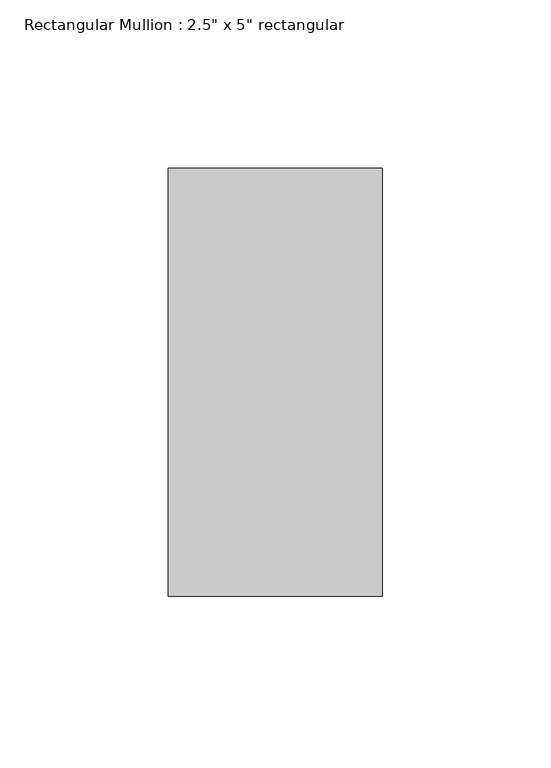
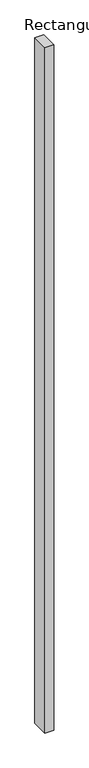
"""IFC4 building model written with IfcOpenShell, lengths in millimetres: member geometry."""

from ifc_helpers import new_model, si_unit, frame, origin, place, context, project, spatial, polyline, outline, extrude, source, transform, mapped, element, save


def member_ca95d35f(model_context):
    return source(origin(), model_context, "Body", "SweptSolid", [
        extrude(outline(polyline([(0.0, 63.5), (0.0, -63.5), (-63.5, -63.5), (-63.5, 63.5), (0.0, 63.5)])), frame((0.0, 0.0, -5295.9), z_axis=(0.0, 0.0, 1.0), x_axis=(1.0, 0.0, 0.0)), (0.0, 0.0, 1.0), 5295.9),
    ])


if __name__ == "__main__":
    model = new_model("IFC4")
    model_context = context("Model", 3, world=origin())
    ifc_project = project(units=[si_unit("LENGTHUNIT", "METRE", prefix="MILLI")], contexts=[model_context])
    site = spatial("IfcSite", under=ifc_project)
    building = spatial("IfcBuilding", under=site)
    placement = place(None, origin())
    member_shape = member_ca95d35f(model_context)
    element("IfcMember", 1, ObjectType="Rectangular Mullion : 2.5\" x 5\" rectangular", at=placement, inside=building, context=model_context, shape_type="MappedRepresentation", body=[
        mapped(member_shape, transform((0.0, 0.0, 0.0), x_axis=(1.0, 0.0, 0.0), y_axis=(0.0, 1.0, 0.0), z_axis=(0.0, 0.0, 1.0))),
    ])
    save(model, "model.ifc")

# Revit data of these elements
# Type "Rectangular Mullion : 2.5\" x 5\" rectangular"
#   built-in parameter 1007304 = 0.416667 (stored number, unit not read)
#   built-in parameter 1007301 = 0.104167 (stored number, unit not read)
#   built-in parameter 1007300 = 0.104167 (stored number, unit not read)
# Element 1 (IfcMember, "Rectangular Mullion : 2.5\" x 5\" rectangular")
#   Materials on its faces: "Aluminum"
# Materials
#   "Aluminum": class "Metal", colour RGB 247 247 247, transparency 0, Description = "Aluminum 6061", Cost = 0
